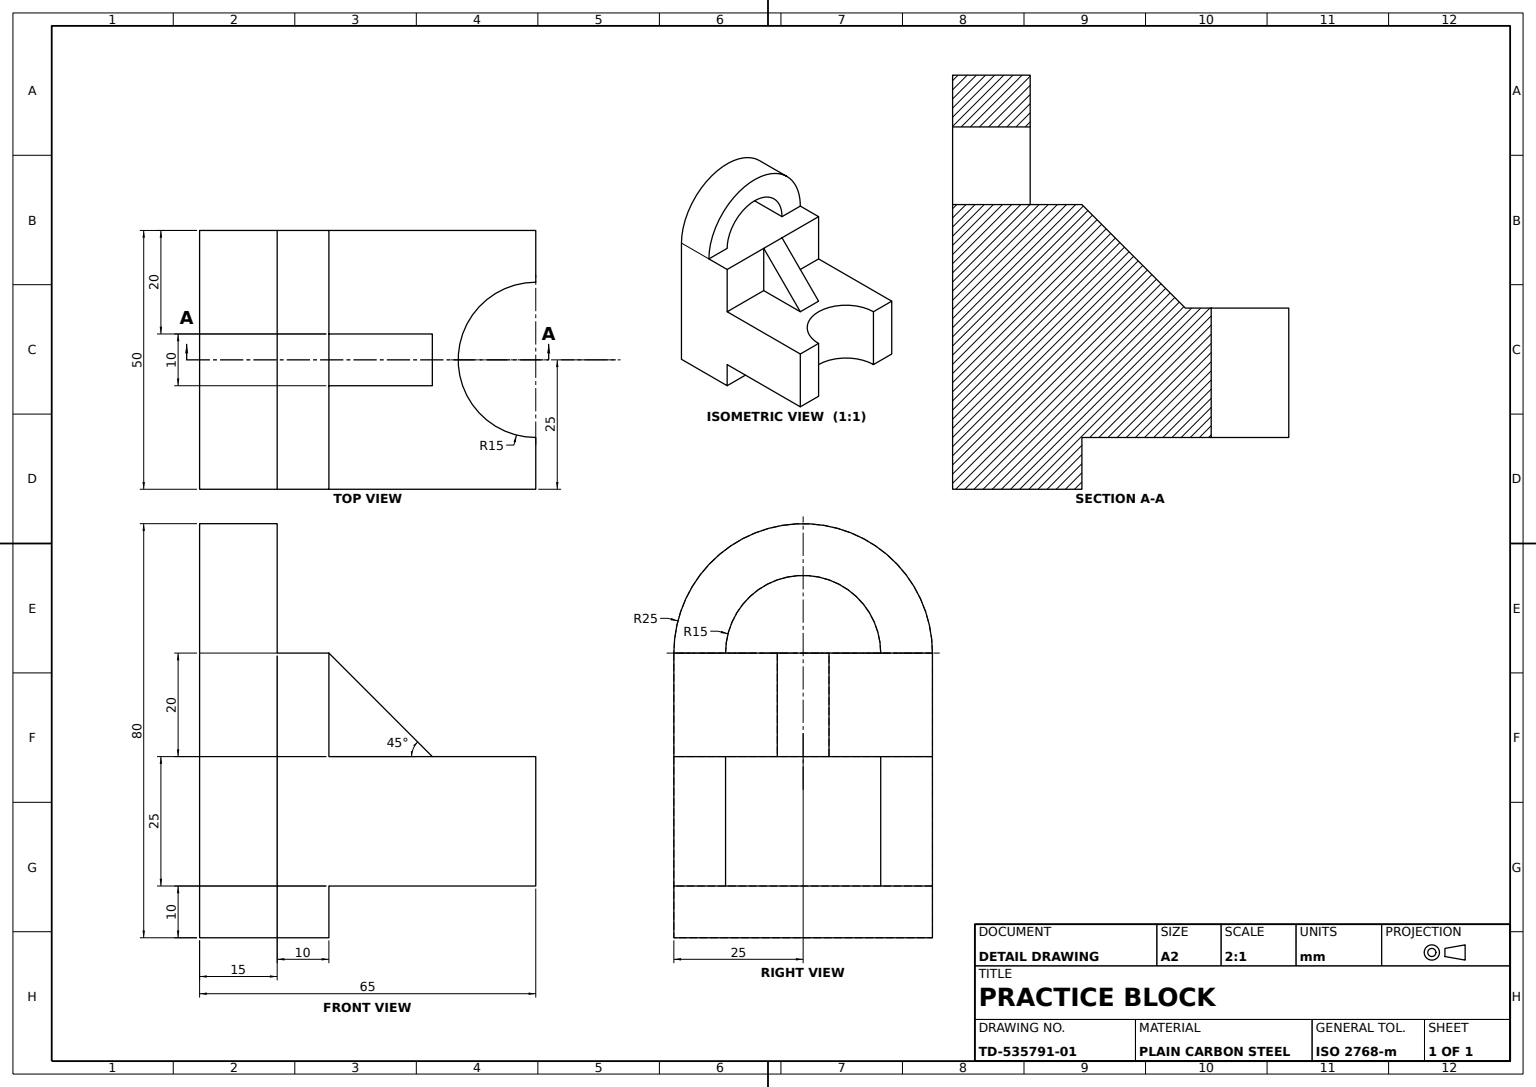
SolidWorks part; units mm, degrees
material "Plain Carbon Steel"
ref_plane "Front Plane" through (0, 0, 0) normal (0, 0, 1) x (1, 0, 0)
ref_plane "Top Plane" through (0, 0, 0) normal (0, 1, 0) x (1, 0, 0)
ref_plane "Right Plane" through (0, 0, 0) normal (1, 0, 0) x (0, 0, -1)
sketch "Base Block Profile" plane through (0, 0, 0) normal (0, 0, 1) x (1, 0, 0)
  line L0 (0, 0) -> (65, 0)
  line L1 (65, 0) -> (65, 25)
  line L2 (65, 25) -> (0, 25)
  line L3 (0, 25) -> (0, 0)
  dimension "D1" = 65
  dimension "D2" = 25
extrude "Base Block 65x25x50" add sketch "Base Block Profile" against normal blind 50
sketch "Upright Profile" plane through (0, 0, 0) normal (-1, 0, 0) x (0, 0, 1)
  line L0 (-50, 25) -> (-50, 45)
  line L1 (-50, 45) -> (0, 45)
  line L2 (0, 45) -> (0, 25)
  line L3 (-50, 25) -> (0, 25)
  dimension "D1" = 20
extrude "Upright Block" add sketch "Upright Profile" against normal blind 25
sketch "Bottom Tongue Profile" plane through (0, 0, 0) normal (0, 0, 1) x (1, 0, 0)
  line L0 (0, 0) -> (0, -10)
  line L1 (0, -10) -> (25, -10)
  line L2 (25, -10) -> (25, 0)
  line L3 (0, 0) -> (65, 0) construction
  line L4 (25, 0) -> (0, 0)
  dimension "D1" = 10
  dimension "D2" = 25
extrude "Bottom Tongue 10x25" add sketch "Bottom Tongue Profile" against normal blind 50
sketch "End Notch Profile" plane through (0, 25, 0) normal (0, 1, 0) x (1, 0, 0)
  line L0 (65, 50) -> (65, 0) construction
  circle A0 centre (65, 25) radius 15
  dimension "D1" = 15
extrude "Round End Notch" cut sketch "End Notch Profile" against normal blind 50
sketch "Top Boss Profile" plane through (0, 0, 0) normal (-1, 0, 0) x (0, 0, 1)
  line L0 (0, 45) -> (-50, 45) construction
  circle A0 centre (-25, 45) radius 25
  dimension "D1" = 25
extrude "Rounded Top Boss" add sketch "Top Boss Profile" against normal blind 15
sketch "Boss Hole Profile" plane through (15, 0, 0) normal (1, 0, 0) x (0, 0, -1)
  line L0 (50, 45) -> (0, 45) construction
  line L1 (10, 45) -> (40, 45)
  arc A0 (40, 45) -> (10, 45) centre (25, 45) ccw
  dimension "D1" = 15
extrude "Boss Half Hole Ø15" cut sketch "Boss Hole Profile" against normal blind 15
sketch "Support Wedge Profile" plane through (0, 0, 0) normal (0, 0, 1) x (1, 0, 0)
  line L0 (25, 45) -> (25, 25)
  line L1 (25, 25) -> (45, 25)
  line L2 (65, 25) -> (25, 25) construction
  line L3 (45, 25) -> (25, 45)
extrude "Support Wedge" add sketch "Support Wedge Profile" against normal blind 50
sketch "Rib Trim Front Profile" plane through (0, 0, 0) normal (0, 0, 1) x (1, 0, 0)
  line L0 (25, 45) -> (45, 25)
  line L1 (45, 25) -> (25, 25)
  line L2 (25, 25) -> (25, 45)
  dimension "D1" = 20
extrude "Rib Trim Front" cut sketch "Rib Trim Front Profile" against normal blind 20
sketch "Rib Trim Rear Profile" plane through (0, 0, -50) normal (0, 0, -1) x (-1, 0, 0)
  line L0 (-25, 45) -> (-25, 25)
  line L1 (-25, 25) -> (-45, 25)
  line L4 (-45, 25) -> (-25, 45)
  line L5 (-65, 0) -> (-65, 25) construction
  dimension "D1" = 20
  dimension "D2" = 20
  dimension "D3" = 20
  dimension "D4" = 90
extrude "Rib Trim Rear" cut sketch "Rib Trim Rear Profile" against normal blind 20
